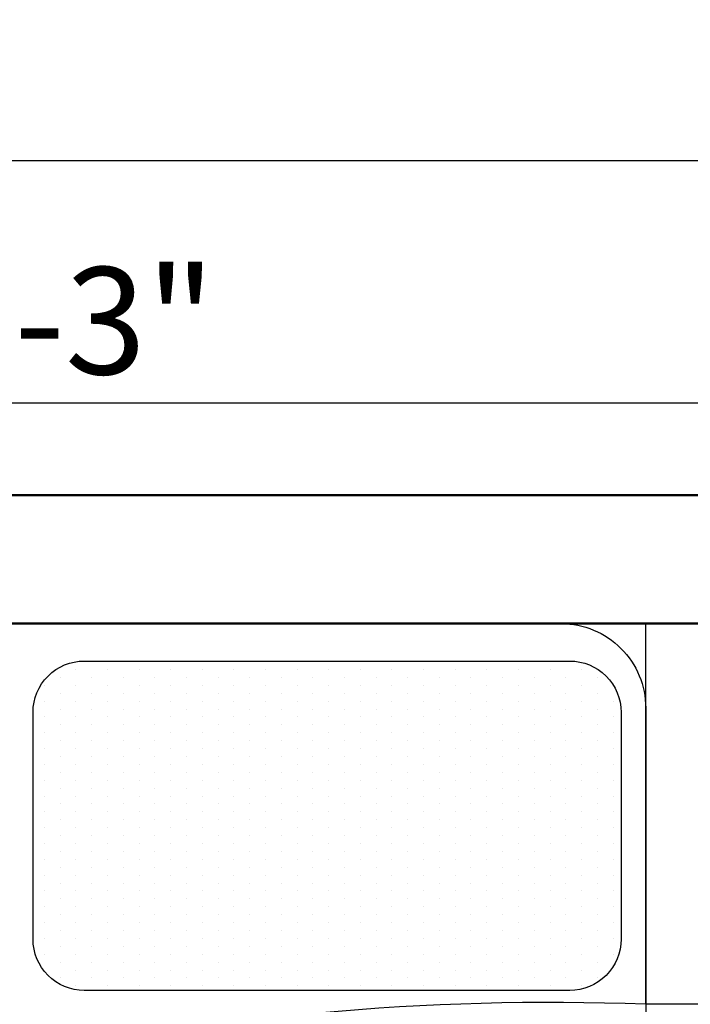
# Model space of a CAD drawing. Units: inches. Extents: x 3064 to 19385, y 846 to 15425.
# Tile 78 of 108: x 6708 to 6739, y 1964 to 2010. Entities that reach past the tile are written whole.
import ezdxf

# ---------------------------------------------------------------- set-up
doc = ezdxf.new("R2010")
doc.units = ezdxf.units.IN
for name, color, linetype, lineweight in [('A-ANNO-DIMS', 2, 'Continuous', 18), ('A-FLOR-FIXT', 9, 'Continuous', 18), ('A-WALL', 7, 'Continuous', 50)]:
    doc.layers.add(name, color=color, linetype=linetype, lineweight=lineweight)
doc.layers.add('BLOCK', color=6, linetype='Continuous')
doc.styles.get("Standard").update_dxf_attribs({"font": 'arial.ttf'})
doc.dimstyles.new('ISO-25', dxfattribs={"dimtxt": 9, "dimasz": 2.5, "dimexe": 1.25, "dimexo": 0.625, "dimtad": 1, "dimdec": 1, "dimlunit": 3, "dimtxsty": 'Standard', "dimcen": 2.5, "dimadec": 0, "dimazin": 0, "dimtfac": 1, "dimtdec": 1, "dimtmove": 0, "dimatfit": 3, "dimfxl": 1, "dimarcsym": 0})

# ---------------------------------------------------------------- blocks, each defined once
blk = doc.blocks.new('*X7')
at = {"color": 0}
for p, q in [((273.9375, 457.03125), (273.9375, 457.03125)), ((274.3125, 457.03125), (274.3125, 457.03125)), ((274.6875, 457.03125), (274.6875, 457.03125)), ((275.0625, 457.03125), (275.0625, 457.03125)), ((275.4375, 457.03125), (275.4375, 457.03125)), ((275.8125, 457.03125), (275.8125, 457.03125)), ((276.1875, 457.03125), (276.1875, 457.03125)), ((276.5625, 457.03125), (276.5625, 457.03125)), ((276.9375, 457.03125), (276.9375, 457.03125)), ((277.3125, 457.03125), (277.3125, 457.03125)), ((277.6875, 457.03125), (277.6875, 457.03125)), ((278.0625, 457.03125), (278.0625, 457.03125)), ((278.4375, 457.03125), (278.4375, 457.03125)), ((278.8125, 457.03125), (278.8125, 457.03125)), ((279.1875, 457.03125), (279.1875, 457.03125)), ((279.5625, 457.03125), (279.5625, 457.03125)), ((273.75, 456.9375), (273.75, 456.9375)), ((274.125, 456.9375), (274.125, 456.9375)), ((274.5, 456.9375), (274.5, 456.9375)), ((274.875, 456.9375), (274.875, 456.9375)), ((275.25, 456.9375), (275.25, 456.9375)), ((275.625, 456.9375), (275.625, 456.9375)), ((276, 456.9375), (276, 456.9375)), ((276.375, 456.9375), (276.375, 456.9375)), ((276.75, 456.9375), (276.75, 456.9375)), ((277.125, 456.9375), (277.125, 456.9375)), ((277.5, 456.9375), (277.5, 456.9375)), ((277.875, 456.9375), (277.875, 456.9375)), ((278.25, 456.9375), (278.25, 456.9375)), ((278.625, 456.9375), (278.625, 456.9375)), ((279, 456.9375), (279, 456.9375)), ((279.375, 456.9375), (279.375, 456.9375)), ((279.75, 456.9375), (279.75, 456.9375)), ((273.375, 456.75), (273.375, 456.75)), ((273.5625, 456.84375), (273.5625, 456.84375)), ((273.75, 456.75), (273.75, 456.75)), ((273.9375, 456.84375), (273.9375, 456.84375)), ((274.125, 456.75), (274.125, 456.75)), ((274.3125, 456.84375), (274.3125, 456.84375)), ((274.5, 456.75), (274.5, 456.75)), ((274.6875, 456.84375), (274.6875, 456.84375)), ((274.875, 456.75), (274.875, 456.75)), ((275.0625, 456.84375), (275.0625, 456.84375)), ((275.25, 456.75), (275.25, 456.75)), ((275.4375, 456.84375), (275.4375, 456.84375)), ((275.625, 456.75), (275.625, 456.75)), ((275.8125, 456.84375), (275.8125, 456.84375)), ((276, 456.75), (276, 456.75)), ((276.1875, 456.84375), (276.1875, 456.84375)), ((276.375, 456.75), (276.375, 456.75)), ((276.5625, 456.84375), (276.5625, 456.84375)), ((276.75, 456.75), (276.75, 456.75)), ((276.9375, 456.84375), (276.9375, 456.84375)), ((277.125, 456.75), (277.125, 456.75)), ((277.3125, 456.84375), (277.3125, 456.84375)), ((277.5, 456.75), (277.5, 456.75)), ((277.6875, 456.84375), (277.6875, 456.84375)), ((277.875, 456.75), (277.875, 456.75)), ((278.0625, 456.84375), (278.0625, 456.84375)), ((278.25, 456.75), (278.25, 456.75)), ((278.4375, 456.84375), (278.4375, 456.84375)), ((278.625, 456.75), (278.625, 456.75)), ((278.8125, 456.84375), (278.8125, 456.84375)), ((279, 456.75), (279, 456.75)), ((279.1875, 456.84375), (279.1875, 456.84375)), ((279.375, 456.75), (279.375, 456.75)), ((279.5625, 456.84375), (279.5625, 456.84375)), ((279.75, 456.75), (279.75, 456.75)), ((279.9375, 456.84375), (279.9375, 456.84375)), ((280.125, 456.75), (280.125, 456.75)), ((273.5625, 456.65625), (273.5625, 456.65625)), ((273.9375, 456.65625), (273.9375, 456.65625)), ((274.3125, 456.65625), (274.3125, 456.65625)), ((274.6875, 456.65625), (274.6875, 456.65625)), ((275.0625, 456.65625), (275.0625, 456.65625)), ((275.4375, 456.65625), (275.4375, 456.65625)), ((275.8125, 456.65625), (275.8125, 456.65625)), ((276.1875, 456.65625), (276.1875, 456.65625)), ((276.5625, 456.65625), (276.5625, 456.65625)), ((276.9375, 456.65625), (276.9375, 456.65625)), ((277.3125, 456.65625), (277.3125, 456.65625)), ((277.6875, 456.65625), (277.6875, 456.65625)), ((278.0625, 456.65625), (278.0625, 456.65625)), ((278.4375, 456.65625), (278.4375, 456.65625)), ((278.8125, 456.65625), (278.8125, 456.65625)), ((279.1875, 456.65625), (279.1875, 456.65625)), ((279.5625, 456.65625), (279.5625, 456.65625)), ((279.9375, 456.65625), (279.9375, 456.65625)), ((273.375, 456.5625), (273.375, 456.5625)), ((273.75, 456.5625), (273.75, 456.5625)), ((274.125, 456.5625), (274.125, 456.5625)), ((274.5, 456.5625), (274.5, 456.5625)), ((274.875, 456.5625), (274.875, 456.5625)), ((275.25, 456.5625), (275.25, 456.5625)), ((275.625, 456.5625), (275.625, 456.5625)), ((276, 456.5625), (276, 456.5625)), ((276.375, 456.5625), (276.375, 456.5625)), ((276.75, 456.5625), (276.75, 456.5625)), ((277.125, 456.5625), (277.125, 456.5625)), ((277.5, 456.5625), (277.5, 456.5625)), ((277.875, 456.5625), (277.875, 456.5625)), ((278.25, 456.5625), (278.25, 456.5625)), ((278.625, 456.5625), (278.625, 456.5625)), ((279, 456.5625), (279, 456.5625)), ((279.375, 456.5625), (279.375, 456.5625)), ((279.75, 456.5625), (279.75, 456.5625)), ((280.125, 456.5625), (280.125, 456.5625)), ((273.5625, 456.46875), (273.5625, 456.46875)), ((273.9375, 456.46875), (273.9375, 456.46875)), ((274.3125, 456.46875), (274.3125, 456.46875)), ((274.6875, 456.46875), (274.6875, 456.46875)), ((275.0625, 456.46875), (275.0625, 456.46875)), ((275.4375, 456.46875), (275.4375, 456.46875)), ((275.8125, 456.46875), (275.8125, 456.46875)), ((276.1875, 456.46875), (276.1875, 456.46875)), ((276.5625, 456.46875), (276.5625, 456.46875)), ((276.9375, 456.46875), (276.9375, 456.46875)), ((277.3125, 456.46875), (277.3125, 456.46875)), ((277.6875, 456.46875), (277.6875, 456.46875)), ((278.0625, 456.46875), (278.0625, 456.46875)), ((278.4375, 456.46875), (278.4375, 456.46875)), ((278.8125, 456.46875), (278.8125, 456.46875)), ((279.1875, 456.46875), (279.1875, 456.46875)), ((279.5625, 456.46875), (279.5625, 456.46875)), ((279.9375, 456.46875), (279.9375, 456.46875)), ((273.375, 456.375), (273.375, 456.375)), ((273.5625, 456.28125), (273.5625, 456.28125)), ((273.75, 456.375), (273.75, 456.375)), ((273.9375, 456.28125), (273.9375, 456.28125)), ((274.125, 456.375), (274.125, 456.375)), ((274.3125, 456.28125), (274.3125, 456.28125)), ((274.5, 456.375), (274.5, 456.375)), ((274.6875, 456.28125), (274.6875, 456.28125)), ((274.875, 456.375), (274.875, 456.375)), ((275.0625, 456.28125), (275.0625, 456.28125)), ((275.25, 456.375), (275.25, 456.375)), ((275.4375, 456.28125), (275.4375, 456.28125)), ((275.625, 456.375), (275.625, 456.375)), ((275.8125, 456.28125), (275.8125, 456.28125)), ((276, 456.375), (276, 456.375)), ((276.1875, 456.28125), (276.1875, 456.28125)), ((276.375, 456.375), (276.375, 456.375)), ((276.5625, 456.28125), (276.5625, 456.28125)), ((276.75, 456.375), (276.75, 456.375)), ((276.9375, 456.28125), (276.9375, 456.28125)), ((277.125, 456.375), (277.125, 456.375)), ((277.3125, 456.28125), (277.3125, 456.28125)), ((277.5, 456.375), (277.5, 456.375)), ((277.6875, 456.28125), (277.6875, 456.28125)), ((277.875, 456.375), (277.875, 456.375)), ((278.0625, 456.28125), (278.0625, 456.28125)), ((278.25, 456.375), (278.25, 456.375)), ((278.4375, 456.28125), (278.4375, 456.28125)), ((278.625, 456.375), (278.625, 456.375)), ((278.8125, 456.28125), (278.8125, 456.28125)), ((279, 456.375), (279, 456.375)), ((279.1875, 456.28125), (279.1875, 456.28125)), ((279.375, 456.375), (279.375, 456.375)), ((279.5625, 456.28125), (279.5625, 456.28125)), ((279.75, 456.375), (279.75, 456.375)), ((279.9375, 456.28125), (279.9375, 456.28125)), ((280.125, 456.375), (280.125, 456.375)), ((273.375, 456.1875), (273.375, 456.1875)), ((273.75, 456.1875), (273.75, 456.1875)), ((274.125, 456.1875), (274.125, 456.1875)), ((274.5, 456.1875), (274.5, 456.1875)), ((274.875, 456.1875), (274.875, 456.1875)), ((275.25, 456.1875), (275.25, 456.1875)), ((275.625, 456.1875), (275.625, 456.1875)), ((276, 456.1875), (276, 456.1875)), ((276.375, 456.1875), (276.375, 456.1875)), ((276.75, 456.1875), (276.75, 456.1875)), ((277.125, 456.1875), (277.125, 456.1875)), ((277.5, 456.1875), (277.5, 456.1875)), ((277.875, 456.1875), (277.875, 456.1875)), ((278.25, 456.1875), (278.25, 456.1875)), ((278.625, 456.1875), (278.625, 456.1875)), ((279, 456.1875), (279, 456.1875)), ((279.375, 456.1875), (279.375, 456.1875)), ((279.75, 456.1875), (279.75, 456.1875)), ((280.125, 456.1875), (280.125, 456.1875)), ((273.5625, 456.09375), (273.5625, 456.09375)), ((273.9375, 456.09375), (273.9375, 456.09375)), ((274.3125, 456.09375), (274.3125, 456.09375)), ((274.6875, 456.09375), (274.6875, 456.09375)), ((275.0625, 456.09375), (275.0625, 456.09375)), ((275.4375, 456.09375), (275.4375, 456.09375)), ((275.8125, 456.09375), (275.8125, 456.09375)), ((276.1875, 456.09375), (276.1875, 456.09375)), ((276.5625, 456.09375), (276.5625, 456.09375)), ((276.9375, 456.09375), (276.9375, 456.09375)), ((277.3125, 456.09375), (277.3125, 456.09375)), ((277.6875, 456.09375), (277.6875, 456.09375)), ((278.0625, 456.09375), (278.0625, 456.09375)), ((278.4375, 456.09375), (278.4375, 456.09375)), ((278.8125, 456.09375), (278.8125, 456.09375)), ((279.1875, 456.09375), (279.1875, 456.09375)), ((279.5625, 456.09375), (279.5625, 456.09375)), ((279.9375, 456.09375), (279.9375, 456.09375)), ((273.375, 456), (273.375, 456)), ((273.75, 456), (273.75, 456)), ((274.125, 456), (274.125, 456)), ((274.5, 456), (274.5, 456)), ((274.875, 456), (274.875, 456)), ((275.25, 456), (275.25, 456)), ((275.625, 456), (275.625, 456)), ((276, 456), (276, 456)), ((276.375, 456), (276.375, 456)), ((276.75, 456), (276.75, 456)), ((277.125, 456), (277.125, 456)), ((277.5, 456), (277.5, 456)), ((277.875, 456), (277.875, 456)), ((278.25, 456), (278.25, 456)), ((278.625, 456), (278.625, 456)), ((279, 456), (279, 456)), ((279.375, 456), (279.375, 456)), ((279.75, 456), (279.75, 456)), ((280.125, 456), (280.125, 456)), ((273.375, 455.8125), (273.375, 455.8125)), ((273.5625, 455.90625), (273.5625, 455.90625)), ((273.75, 455.8125), (273.75, 455.8125)), ((273.9375, 455.90625), (273.9375, 455.90625)), ((274.125, 455.8125), (274.125, 455.8125)), ((274.3125, 455.90625), (274.3125, 455.90625)), ((274.5, 455.8125), (274.5, 455.8125)), ((274.6875, 455.90625), (274.6875, 455.90625)), ((274.875, 455.8125), (274.875, 455.8125)), ((275.0625, 455.90625), (275.0625, 455.90625)), ((275.25, 455.8125), (275.25, 455.8125)), ((275.4375, 455.90625), (275.4375, 455.90625)), ((275.625, 455.8125), (275.625, 455.8125)), ((275.8125, 455.90625), (275.8125, 455.90625)), ((276, 455.8125), (276, 455.8125)), ((276.1875, 455.90625), (276.1875, 455.90625)), ((276.375, 455.8125), (276.375, 455.8125)), ((276.5625, 455.90625), (276.5625, 455.90625)), ((276.75, 455.8125), (276.75, 455.8125)), ((276.9375, 455.90625), (276.9375, 455.90625)), ((277.125, 455.8125), (277.125, 455.8125)), ((277.3125, 455.90625), (277.3125, 455.90625)), ((277.5, 455.8125), (277.5, 455.8125)), ((277.6875, 455.90625), (277.6875, 455.90625)), ((277.875, 455.8125), (277.875, 455.8125)), ((278.0625, 455.90625), (278.0625, 455.90625)), ((278.25, 455.8125), (278.25, 455.8125)), ((278.4375, 455.90625), (278.4375, 455.90625)), ((278.625, 455.8125), (278.625, 455.8125)), ((278.8125, 455.90625), (278.8125, 455.90625)), ((279, 455.8125), (279, 455.8125)), ((279.1875, 455.90625), (279.1875, 455.90625)), ((279.375, 455.8125), (279.375, 455.8125)), ((279.5625, 455.90625), (279.5625, 455.90625)), ((279.75, 455.8125), (279.75, 455.8125)), ((279.9375, 455.90625), (279.9375, 455.90625)), ((280.125, 455.8125), (280.125, 455.8125)), ((273.5625, 455.71875), (273.5625, 455.71875)), ((273.9375, 455.71875), (273.9375, 455.71875)), ((274.3125, 455.71875), (274.3125, 455.71875)), ((274.6875, 455.71875), (274.6875, 455.71875)), ((275.0625, 455.71875), (275.0625, 455.71875)), ((275.4375, 455.71875), (275.4375, 455.71875)), ((275.8125, 455.71875), (275.8125, 455.71875)), ((276.1875, 455.71875), (276.1875, 455.71875)), ((276.5625, 455.71875), (276.5625, 455.71875)), ((276.9375, 455.71875), (276.9375, 455.71875)), ((277.3125, 455.71875), (277.3125, 455.71875)), ((277.6875, 455.71875), (277.6875, 455.71875)), ((278.0625, 455.71875), (278.0625, 455.71875)), ((278.4375, 455.71875), (278.4375, 455.71875)), ((278.8125, 455.71875), (278.8125, 455.71875)), ((279.1875, 455.71875), (279.1875, 455.71875)), ((279.5625, 455.71875), (279.5625, 455.71875)), ((279.9375, 455.71875), (279.9375, 455.71875)), ((273.375, 455.625), (273.375, 455.625)), ((273.75, 455.625), (273.75, 455.625)), ((274.125, 455.625), (274.125, 455.625)), ((274.5, 455.625), (274.5, 455.625)), ((274.875, 455.625), (274.875, 455.625)), ((275.25, 455.625), (275.25, 455.625)), ((275.625, 455.625), (275.625, 455.625)), ((276, 455.625), (276, 455.625)), ((276.375, 455.625), (276.375, 455.625)), ((276.75, 455.625), (276.75, 455.625)), ((277.125, 455.625), (277.125, 455.625)), ((277.5, 455.625), (277.5, 455.625)), ((277.875, 455.625), (277.875, 455.625)), ((278.25, 455.625), (278.25, 455.625)), ((278.625, 455.625), (278.625, 455.625)), ((279, 455.625), (279, 455.625)), ((279.375, 455.625), (279.375, 455.625)), ((279.75, 455.625), (279.75, 455.625)), ((280.125, 455.625), (280.125, 455.625)), ((273.5625, 455.53125), (273.5625, 455.53125)), ((273.9375, 455.53125), (273.9375, 455.53125)), ((274.3125, 455.53125), (274.3125, 455.53125)), ((274.6875, 455.53125), (274.6875, 455.53125)), ((275.0625, 455.53125), (275.0625, 455.53125)), ((275.4375, 455.53125), (275.4375, 455.53125)), ((275.8125, 455.53125), (275.8125, 455.53125)), ((276.1875, 455.53125), (276.1875, 455.53125)), ((276.5625, 455.53125), (276.5625, 455.53125)), ((276.9375, 455.53125), (276.9375, 455.53125)), ((277.3125, 455.53125), (277.3125, 455.53125)), ((277.6875, 455.53125), (277.6875, 455.53125)), ((278.0625, 455.53125), (278.0625, 455.53125)), ((278.4375, 455.53125), (278.4375, 455.53125)), ((278.8125, 455.53125), (278.8125, 455.53125)), ((279.1875, 455.53125), (279.1875, 455.53125)), ((279.5625, 455.53125), (279.5625, 455.53125)), ((279.9375, 455.53125), (279.9375, 455.53125)), ((273.375, 455.4375), (273.375, 455.4375)), ((273.5625, 455.34375), (273.5625, 455.34375)), ((273.75, 455.4375), (273.75, 455.4375)), ((273.9375, 455.34375), (273.9375, 455.34375)), ((274.125, 455.4375), (274.125, 455.4375)), ((274.3125, 455.34375), (274.3125, 455.34375)), ((274.5, 455.4375), (274.5, 455.4375)), ((274.6875, 455.34375), (274.6875, 455.34375)), ((274.875, 455.4375), (274.875, 455.4375)), ((275.0625, 455.34375), (275.0625, 455.34375)), ((275.25, 455.4375), (275.25, 455.4375)), ((275.4375, 455.34375), (275.4375, 455.34375)), ((275.625, 455.4375), (275.625, 455.4375)), ((275.8125, 455.34375), (275.8125, 455.34375)), ((276, 455.4375), (276, 455.4375)), ((276.1875, 455.34375), (276.1875, 455.34375)), ((276.375, 455.4375), (276.375, 455.4375)), ((276.5625, 455.34375), (276.5625, 455.34375)), ((276.75, 455.4375), (276.75, 455.4375)), ((276.9375, 455.34375), (276.9375, 455.34375)), ((277.125, 455.4375), (277.125, 455.4375)), ((277.3125, 455.34375), (277.3125, 455.34375)), ((277.5, 455.4375), (277.5, 455.4375)), ((277.6875, 455.34375), (277.6875, 455.34375)), ((277.875, 455.4375), (277.875, 455.4375)), ((278.0625, 455.34375), (278.0625, 455.34375)), ((278.25, 455.4375), (278.25, 455.4375)), ((278.4375, 455.34375), (278.4375, 455.34375)), ((278.625, 455.4375), (278.625, 455.4375)), ((278.8125, 455.34375), (278.8125, 455.34375)), ((279, 455.4375), (279, 455.4375)), ((279.1875, 455.34375), (279.1875, 455.34375)), ((279.375, 455.4375), (279.375, 455.4375)), ((279.5625, 455.34375), (279.5625, 455.34375)), ((279.75, 455.4375), (279.75, 455.4375)), ((279.9375, 455.34375), (279.9375, 455.34375)), ((280.125, 455.4375), (280.125, 455.4375)), ((273.375, 455.25), (273.375, 455.25)), ((273.75, 455.25), (273.75, 455.25)), ((274.125, 455.25), (274.125, 455.25)), ((274.5, 455.25), (274.5, 455.25)), ((274.875, 455.25), (274.875, 455.25)), ((275.25, 455.25), (275.25, 455.25)), ((275.625, 455.25), (275.625, 455.25)), ((276, 455.25), (276, 455.25)), ((276.375, 455.25), (276.375, 455.25)), ((276.75, 455.25), (276.75, 455.25)), ((277.125, 455.25), (277.125, 455.25)), ((277.5, 455.25), (277.5, 455.25)), ((277.875, 455.25), (277.875, 455.25)), ((278.25, 455.25), (278.25, 455.25)), ((278.625, 455.25), (278.625, 455.25)), ((279, 455.25), (279, 455.25)), ((279.375, 455.25), (279.375, 455.25)), ((279.75, 455.25), (279.75, 455.25)), ((280.125, 455.25), (280.125, 455.25)), ((273.5625, 455.15625), (273.5625, 455.15625)), ((273.9375, 455.15625), (273.9375, 455.15625)), ((274.3125, 455.15625), (274.3125, 455.15625)), ((274.6875, 455.15625), (274.6875, 455.15625)), ((275.0625, 455.15625), (275.0625, 455.15625)), ((275.4375, 455.15625), (275.4375, 455.15625)), ((275.8125, 455.15625), (275.8125, 455.15625)), ((276.1875, 455.15625), (276.1875, 455.15625)), ((276.5625, 455.15625), (276.5625, 455.15625)), ((276.9375, 455.15625), (276.9375, 455.15625)), ((277.3125, 455.15625), (277.3125, 455.15625)), ((277.6875, 455.15625), (277.6875, 455.15625)), ((278.0625, 455.15625), (278.0625, 455.15625)), ((278.4375, 455.15625), (278.4375, 455.15625)), ((278.8125, 455.15625), (278.8125, 455.15625)), ((279.1875, 455.15625), (279.1875, 455.15625)), ((279.5625, 455.15625), (279.5625, 455.15625)), ((279.9375, 455.15625), (279.9375, 455.15625)), ((273.375, 455.0625), (273.375, 455.0625)), ((273.75, 455.0625), (273.75, 455.0625)), ((274.125, 455.0625), (274.125, 455.0625)), ((274.5, 455.0625), (274.5, 455.0625)), ((274.875, 455.0625), (274.875, 455.0625)), ((275.25, 455.0625), (275.25, 455.0625)), ((275.625, 455.0625), (275.625, 455.0625)), ((276, 455.0625), (276, 455.0625)), ((276.375, 455.0625), (276.375, 455.0625)), ((276.75, 455.0625), (276.75, 455.0625)), ((277.125, 455.0625), (277.125, 455.0625)), ((277.5, 455.0625), (277.5, 455.0625)), ((277.875, 455.0625), (277.875, 455.0625)), ((278.25, 455.0625), (278.25, 455.0625)), ((278.625, 455.0625), (278.625, 455.0625)), ((279, 455.0625), (279, 455.0625)), ((279.375, 455.0625), (279.375, 455.0625)), ((279.75, 455.0625), (279.75, 455.0625)), ((280.125, 455.0625), (280.125, 455.0625)), ((273.375, 454.875), (273.375, 454.875)), ((273.5625, 454.96875), (273.5625, 454.96875)), ((273.75, 454.875), (273.75, 454.875)), ((273.9375, 454.96875), (273.9375, 454.96875)), ((274.125, 454.875), (274.125, 454.875)), ((274.3125, 454.96875), (274.3125, 454.96875)), ((274.5, 454.875), (274.5, 454.875)), ((274.6875, 454.96875), (274.6875, 454.96875)), ((274.875, 454.875), (274.875, 454.875)), ((275.0625, 454.96875), (275.0625, 454.96875)), ((275.25, 454.875), (275.25, 454.875)), ((275.4375, 454.96875), (275.4375, 454.96875)), ((275.625, 454.875), (275.625, 454.875)), ((275.8125, 454.96875), (275.8125, 454.96875)), ((276, 454.875), (276, 454.875)), ((276.1875, 454.96875), (276.1875, 454.96875)), ((276.375, 454.875), (276.375, 454.875)), ((276.5625, 454.96875), (276.5625, 454.96875)), ((276.75, 454.875), (276.75, 454.875)), ((276.9375, 454.96875), (276.9375, 454.96875)), ((277.125, 454.875), (277.125, 454.875)), ((277.3125, 454.96875), (277.3125, 454.96875)), ((277.5, 454.875), (277.5, 454.875)), ((277.6875, 454.96875), (277.6875, 454.96875)), ((277.875, 454.875), (277.875, 454.875)), ((278.0625, 454.96875), (278.0625, 454.96875)), ((278.25, 454.875), (278.25, 454.875)), ((278.4375, 454.96875), (278.4375, 454.96875)), ((278.625, 454.875), (278.625, 454.875)), ((278.8125, 454.96875), (278.8125, 454.96875)), ((279, 454.875), (279, 454.875)), ((279.1875, 454.96875), (279.1875, 454.96875)), ((279.375, 454.875), (279.375, 454.875)), ((279.5625, 454.96875), (279.5625, 454.96875)), ((279.75, 454.875), (279.75, 454.875)), ((279.9375, 454.96875), (279.9375, 454.96875)), ((280.125, 454.875), (280.125, 454.875)), ((273.5625, 454.78125), (273.5625, 454.78125)), ((273.9375, 454.78125), (273.9375, 454.78125)), ((274.3125, 454.78125), (274.3125, 454.78125)), ((274.6875, 454.78125), (274.6875, 454.78125)), ((275.0625, 454.78125), (275.0625, 454.78125)), ((275.4375, 454.78125), (275.4375, 454.78125)), ((275.8125, 454.78125), (275.8125, 454.78125)), ((276.1875, 454.78125), (276.1875, 454.78125)), ((276.5625, 454.78125), (276.5625, 454.78125)), ((276.9375, 454.78125), (276.9375, 454.78125)), ((277.3125, 454.78125), (277.3125, 454.78125)), ((277.6875, 454.78125), (277.6875, 454.78125)), ((278.0625, 454.78125), (278.0625, 454.78125)), ((278.4375, 454.78125), (278.4375, 454.78125)), ((278.8125, 454.78125), (278.8125, 454.78125)), ((279.1875, 454.78125), (279.1875, 454.78125)), ((279.5625, 454.78125), (279.5625, 454.78125)), ((279.9375, 454.78125), (279.9375, 454.78125)), ((273.375, 454.6875), (273.375, 454.6875)), ((273.75, 454.6875), (273.75, 454.6875)), ((274.125, 454.6875), (274.125, 454.6875)), ((274.5, 454.6875), (274.5, 454.6875)), ((274.875, 454.6875), (274.875, 454.6875)), ((275.25, 454.6875), (275.25, 454.6875)), ((275.625, 454.6875), (275.625, 454.6875)), ((276, 454.6875), (276, 454.6875)), ((276.375, 454.6875), (276.375, 454.6875)), ((276.75, 454.6875), (276.75, 454.6875)), ((277.125, 454.6875), (277.125, 454.6875)), ((277.5, 454.6875), (277.5, 454.6875)), ((277.875, 454.6875), (277.875, 454.6875)), ((278.25, 454.6875), (278.25, 454.6875)), ((278.625, 454.6875), (278.625, 454.6875)), ((279, 454.6875), (279, 454.6875)), ((279.375, 454.6875), (279.375, 454.6875)), ((279.75, 454.6875), (279.75, 454.6875)), ((280.125, 454.6875), (280.125, 454.6875)), ((273.5625, 454.59375), (273.5625, 454.59375)), ((273.9375, 454.59375), (273.9375, 454.59375)), ((274.3125, 454.59375), (274.3125, 454.59375)), ((274.6875, 454.59375), (274.6875, 454.59375)), ((275.0625, 454.59375), (275.0625, 454.59375)), ((275.4375, 454.59375), (275.4375, 454.59375)), ((275.8125, 454.59375), (275.8125, 454.59375)), ((276.1875, 454.59375), (276.1875, 454.59375)), ((276.5625, 454.59375), (276.5625, 454.59375)), ((276.9375, 454.59375), (276.9375, 454.59375)), ((277.3125, 454.59375), (277.3125, 454.59375)), ((277.6875, 454.59375), (277.6875, 454.59375)), ((278.0625, 454.59375), (278.0625, 454.59375)), ((278.4375, 454.59375), (278.4375, 454.59375)), ((278.8125, 454.59375), (278.8125, 454.59375)), ((279.1875, 454.59375), (279.1875, 454.59375)), ((279.5625, 454.59375), (279.5625, 454.59375)), ((279.9375, 454.59375), (279.9375, 454.59375)), ((273.375, 454.5), (273.375, 454.5)), ((273.5625, 454.40625), (273.5625, 454.40625)), ((273.75, 454.5), (273.75, 454.5)), ((273.9375, 454.40625), (273.9375, 454.40625)), ((274.125, 454.5), (274.125, 454.5)), ((274.3125, 454.40625), (274.3125, 454.40625)), ((274.5, 454.5), (274.5, 454.5)), ((274.6875, 454.40625), (274.6875, 454.40625)), ((274.875, 454.5), (274.875, 454.5)), ((275.0625, 454.40625), (275.0625, 454.40625)), ((275.25, 454.5), (275.25, 454.5)), ((275.4375, 454.40625), (275.4375, 454.40625)), ((275.625, 454.5), (275.625, 454.5)), ((275.8125, 454.40625), (275.8125, 454.40625)), ((276, 454.5), (276, 454.5)), ((276.1875, 454.40625), (276.1875, 454.40625)), ((276.375, 454.5), (276.375, 454.5)), ((276.5625, 454.40625), (276.5625, 454.40625)), ((276.75, 454.5), (276.75, 454.5)), ((276.9375, 454.40625), (276.9375, 454.40625)), ((277.125, 454.5), (277.125, 454.5)), ((277.3125, 454.40625), (277.3125, 454.40625)), ((277.5, 454.5), (277.5, 454.5)), ((277.6875, 454.40625), (277.6875, 454.40625)), ((277.875, 454.5), (277.875, 454.5)), ((278.0625, 454.40625), (278.0625, 454.40625)), ((278.25, 454.5), (278.25, 454.5)), ((278.4375, 454.40625), (278.4375, 454.40625)), ((278.625, 454.5), (278.625, 454.5)), ((278.8125, 454.40625), (278.8125, 454.40625)), ((279, 454.5), (279, 454.5)), ((279.1875, 454.40625), (279.1875, 454.40625)), ((279.375, 454.5), (279.375, 454.5)), ((279.5625, 454.40625), (279.5625, 454.40625)), ((279.75, 454.5), (279.75, 454.5)), ((279.9375, 454.40625), (279.9375, 454.40625)), ((280.125, 454.5), (280.125, 454.5)), ((273.375, 454.3125), (273.375, 454.3125)), ((273.75, 454.3125), (273.75, 454.3125)), ((274.125, 454.3125), (274.125, 454.3125)), ((274.5, 454.3125), (274.5, 454.3125)), ((274.875, 454.3125), (274.875, 454.3125)), ((275.25, 454.3125), (275.25, 454.3125)), ((275.625, 454.3125), (275.625, 454.3125)), ((276, 454.3125), (276, 454.3125)), ((276.375, 454.3125), (276.375, 454.3125)), ((276.75, 454.3125), (276.75, 454.3125)), ((277.125, 454.3125), (277.125, 454.3125)), ((277.5, 454.3125), (277.5, 454.3125)), ((277.875, 454.3125), (277.875, 454.3125)), ((278.25, 454.3125), (278.25, 454.3125)), ((278.625, 454.3125), (278.625, 454.3125)), ((279, 454.3125), (279, 454.3125)), ((279.375, 454.3125), (279.375, 454.3125)), ((279.75, 454.3125), (279.75, 454.3125)), ((280.125, 454.3125), (280.125, 454.3125)), ((273.5625, 454.21875), (273.5625, 454.21875)), ((273.9375, 454.21875), (273.9375, 454.21875)), ((274.3125, 454.21875), (274.3125, 454.21875)), ((274.6875, 454.21875), (274.6875, 454.21875)), ((275.0625, 454.21875), (275.0625, 454.21875)), ((275.4375, 454.21875), (275.4375, 454.21875)), ((275.8125, 454.21875), (275.8125, 454.21875)), ((276.1875, 454.21875), (276.1875, 454.21875)), ((276.5625, 454.21875), (276.5625, 454.21875)), ((276.9375, 454.21875), (276.9375, 454.21875)), ((277.3125, 454.21875), (277.3125, 454.21875)), ((277.6875, 454.21875), (277.6875, 454.21875)), ((278.0625, 454.21875), (278.0625, 454.21875)), ((278.4375, 454.21875), (278.4375, 454.21875)), ((278.8125, 454.21875), (278.8125, 454.21875)), ((279.1875, 454.21875), (279.1875, 454.21875)), ((279.5625, 454.21875), (279.5625, 454.21875)), ((279.9375, 454.21875), (279.9375, 454.21875)), ((273.375, 454.125), (273.375, 454.125)), ((273.75, 454.125), (273.75, 454.125)), ((274.125, 454.125), (274.125, 454.125)), ((274.5, 454.125), (274.5, 454.125)), ((274.875, 454.125), (274.875, 454.125)), ((275.25, 454.125), (275.25, 454.125)), ((275.625, 454.125), (275.625, 454.125)), ((276, 454.125), (276, 454.125)), ((276.375, 454.125), (276.375, 454.125)), ((276.75, 454.125), (276.75, 454.125)), ((277.125, 454.125), (277.125, 454.125)), ((277.5, 454.125), (277.5, 454.125)), ((277.875, 454.125), (277.875, 454.125)), ((278.25, 454.125), (278.25, 454.125)), ((278.625, 454.125), (278.625, 454.125)), ((279, 454.125), (279, 454.125)), ((279.375, 454.125), (279.375, 454.125)), ((279.75, 454.125), (279.75, 454.125)), ((280.125, 454.125), (280.125, 454.125)), ((273.375, 453.9375), (273.375, 453.9375)), ((273.5625, 454.03125), (273.5625, 454.03125)), ((273.75, 453.9375), (273.75, 453.9375)), ((273.9375, 454.03125), (273.9375, 454.03125)), ((274.125, 453.9375), (274.125, 453.9375)), ((274.3125, 454.03125), (274.3125, 454.03125)), ((274.5, 453.9375), (274.5, 453.9375)), ((274.6875, 454.03125), (274.6875, 454.03125)), ((274.875, 453.9375), (274.875, 453.9375)), ((275.0625, 454.03125), (275.0625, 454.03125)), ((275.25, 453.9375), (275.25, 453.9375)), ((275.4375, 454.03125), (275.4375, 454.03125)), ((275.625, 453.9375), (275.625, 453.9375)), ((275.8125, 454.03125), (275.8125, 454.03125)), ((276, 453.9375), (276, 453.9375)), ((276.1875, 454.03125), (276.1875, 454.03125)), ((276.375, 453.9375), (276.375, 453.9375)), ((276.5625, 454.03125), (276.5625, 454.03125)), ((276.75, 453.9375), (276.75, 453.9375)), ((276.9375, 454.03125), (276.9375, 454.03125)), ((277.125, 453.9375), (277.125, 453.9375)), ((277.3125, 454.03125), (277.3125, 454.03125)), ((277.5, 453.9375), (277.5, 453.9375)), ((277.6875, 454.03125), (277.6875, 454.03125)), ((277.875, 453.9375), (277.875, 453.9375)), ((278.0625, 454.03125), (278.0625, 454.03125)), ((278.25, 453.9375), (278.25, 453.9375)), ((278.4375, 454.03125), (278.4375, 454.03125)), ((278.625, 453.9375), (278.625, 453.9375)), ((278.8125, 454.03125), (278.8125, 454.03125)), ((279, 453.9375), (279, 453.9375)), ((279.1875, 454.03125), (279.1875, 454.03125)), ((279.375, 453.9375), (279.375, 453.9375)), ((279.5625, 454.03125), (279.5625, 454.03125)), ((279.75, 453.9375), (279.75, 453.9375)), ((279.9375, 454.03125), (279.9375, 454.03125)), ((280.125, 453.9375), (280.125, 453.9375)), ((273.5625, 453.84375), (273.5625, 453.84375)), ((273.9375, 453.84375), (273.9375, 453.84375)), ((274.3125, 453.84375), (274.3125, 453.84375)), ((274.6875, 453.84375), (274.6875, 453.84375)), ((275.0625, 453.84375), (275.0625, 453.84375)), ((275.4375, 453.84375), (275.4375, 453.84375)), ((275.8125, 453.84375), (275.8125, 453.84375)), ((276.1875, 453.84375), (276.1875, 453.84375)), ((276.5625, 453.84375), (276.5625, 453.84375)), ((276.9375, 453.84375), (276.9375, 453.84375)), ((277.3125, 453.84375), (277.3125, 453.84375)), ((277.6875, 453.84375), (277.6875, 453.84375)), ((278.0625, 453.84375), (278.0625, 453.84375)), ((278.4375, 453.84375), (278.4375, 453.84375)), ((278.8125, 453.84375), (278.8125, 453.84375)), ((279.1875, 453.84375), (279.1875, 453.84375)), ((279.5625, 453.84375), (279.5625, 453.84375)), ((279.9375, 453.84375), (279.9375, 453.84375)), ((273.375, 453.75), (273.375, 453.75)), ((273.75, 453.75), (273.75, 453.75)), ((274.125, 453.75), (274.125, 453.75)), ((274.5, 453.75), (274.5, 453.75)), ((274.875, 453.75), (274.875, 453.75)), ((275.25, 453.75), (275.25, 453.75)), ((275.625, 453.75), (275.625, 453.75)), ((276, 453.75), (276, 453.75)), ((276.375, 453.75), (276.375, 453.75)), ((276.75, 453.75), (276.75, 453.75)), ((277.125, 453.75), (277.125, 453.75)), ((277.5, 453.75), (277.5, 453.75)), ((277.875, 453.75), (277.875, 453.75)), ((278.25, 453.75), (278.25, 453.75)), ((278.625, 453.75), (278.625, 453.75)), ((279, 453.75), (279, 453.75)), ((279.375, 453.75), (279.375, 453.75)), ((279.75, 453.75), (279.75, 453.75)), ((280.125, 453.75), (280.125, 453.75)), ((273.5625, 453.65625), (273.5625, 453.65625)), ((273.9375, 453.65625), (273.9375, 453.65625)), ((274.3125, 453.65625), (274.3125, 453.65625)), ((274.6875, 453.65625), (274.6875, 453.65625)), ((275.0625, 453.65625), (275.0625, 453.65625)), ((275.4375, 453.65625), (275.4375, 453.65625)), ((275.8125, 453.65625), (275.8125, 453.65625)), ((276.1875, 453.65625), (276.1875, 453.65625)), ((276.5625, 453.65625), (276.5625, 453.65625)), ((276.9375, 453.65625), (276.9375, 453.65625)), ((277.3125, 453.65625), (277.3125, 453.65625)), ((277.6875, 453.65625), (277.6875, 453.65625)), ((278.0625, 453.65625), (278.0625, 453.65625)), ((278.4375, 453.65625), (278.4375, 453.65625)), ((278.8125, 453.65625), (278.8125, 453.65625)), ((279.1875, 453.65625), (279.1875, 453.65625)), ((279.5625, 453.65625), (279.5625, 453.65625)), ((279.9375, 453.65625), (279.9375, 453.65625)), ((273.375, 453.5625), (273.375, 453.5625)), ((273.5625, 453.46875), (273.5625, 453.46875)), ((273.75, 453.5625), (273.75, 453.5625)), ((273.9375, 453.46875), (273.9375, 453.46875)), ((274.125, 453.5625), (274.125, 453.5625)), ((274.3125, 453.46875), (274.3125, 453.46875)), ((274.5, 453.5625), (274.5, 453.5625)), ((274.6875, 453.46875), (274.6875, 453.46875)), ((274.875, 453.5625), (274.875, 453.5625)), ((275.0625, 453.46875), (275.0625, 453.46875)), ((275.25, 453.5625), (275.25, 453.5625)), ((275.4375, 453.46875), (275.4375, 453.46875)), ((275.625, 453.5625), (275.625, 453.5625)), ((275.8125, 453.46875), (275.8125, 453.46875)), ((276, 453.5625), (276, 453.5625)), ((276.1875, 453.46875), (276.1875, 453.46875)), ((276.375, 453.5625), (276.375, 453.5625)), ((276.5625, 453.46875), (276.5625, 453.46875)), ((276.75, 453.5625), (276.75, 453.5625)), ((276.9375, 453.46875), (276.9375, 453.46875)), ((277.125, 453.5625), (277.125, 453.5625)), ((277.3125, 453.46875), (277.3125, 453.46875)), ((277.5, 453.5625), (277.5, 453.5625)), ((277.6875, 453.46875), (277.6875, 453.46875)), ((277.875, 453.5625), (277.875, 453.5625)), ((278.0625, 453.46875), (278.0625, 453.46875)), ((278.25, 453.5625), (278.25, 453.5625)), ((278.4375, 453.46875), (278.4375, 453.46875)), ((278.625, 453.5625), (278.625, 453.5625)), ((278.8125, 453.46875), (278.8125, 453.46875)), ((279, 453.5625), (279, 453.5625)), ((279.1875, 453.46875), (279.1875, 453.46875)), ((279.375, 453.5625), (279.375, 453.5625)), ((279.5625, 453.46875), (279.5625, 453.46875)), ((279.75, 453.5625), (279.75, 453.5625)), ((279.9375, 453.46875), (279.9375, 453.46875)), ((280.125, 453.5625), (280.125, 453.5625)), ((273.375, 453.375), (273.375, 453.375)), ((273.75, 453.375), (273.75, 453.375)), ((274.125, 453.375), (274.125, 453.375)), ((274.5, 453.375), (274.5, 453.375)), ((274.875, 453.375), (274.875, 453.375)), ((275.25, 453.375), (275.25, 453.375)), ((275.625, 453.375), (275.625, 453.375)), ((276, 453.375), (276, 453.375)), ((276.375, 453.375), (276.375, 453.375)), ((276.75, 453.375), (276.75, 453.375)), ((277.125, 453.375), (277.125, 453.375)), ((277.5, 453.375), (277.5, 453.375)), ((277.875, 453.375), (277.875, 453.375)), ((278.25, 453.375), (278.25, 453.375)), ((278.625, 453.375), (278.625, 453.375)), ((279, 453.375), (279, 453.375)), ((279.375, 453.375), (279.375, 453.375)), ((279.75, 453.375), (279.75, 453.375)), ((273.5625, 453.28125), (273.5625, 453.28125)), ((273.9375, 453.28125), (273.9375, 453.28125)), ((274.3125, 453.28125), (274.3125, 453.28125)), ((274.6875, 453.28125), (274.6875, 453.28125)), ((275.0625, 453.28125), (275.0625, 453.28125)), ((275.4375, 453.28125), (275.4375, 453.28125)), ((275.8125, 453.28125), (275.8125, 453.28125)), ((276.1875, 453.28125), (276.1875, 453.28125)), ((276.5625, 453.28125), (276.5625, 453.28125)), ((276.9375, 453.28125), (276.9375, 453.28125)), ((277.3125, 453.28125), (277.3125, 453.28125)), ((277.6875, 453.28125), (277.6875, 453.28125)), ((278.0625, 453.28125), (278.0625, 453.28125)), ((278.4375, 453.28125), (278.4375, 453.28125)), ((278.8125, 453.28125), (278.8125, 453.28125)), ((279.1875, 453.28125), (279.1875, 453.28125)), ((279.5625, 453.28125), (279.5625, 453.28125)), ((279.9375, 453.28125), (279.9375, 453.28125)), ((273.75, 453.1875), (273.75, 453.1875)), ((274.125, 453.1875), (274.125, 453.1875)), ((274.5, 453.1875), (274.5, 453.1875)), ((274.875, 453.1875), (274.875, 453.1875)), ((275.25, 453.1875), (275.25, 453.1875)), ((275.625, 453.1875), (275.625, 453.1875)), ((276, 453.1875), (276, 453.1875)), ((276.375, 453.1875), (276.375, 453.1875)), ((276.75, 453.1875), (276.75, 453.1875)), ((277.125, 453.1875), (277.125, 453.1875)), ((277.5, 453.1875), (277.5, 453.1875)), ((277.875, 453.1875), (277.875, 453.1875)), ((278.25, 453.1875), (278.25, 453.1875)), ((278.625, 453.1875), (278.625, 453.1875)), ((279, 453.1875), (279, 453.1875)), ((279.375, 453.1875), (279.375, 453.1875)), ((279.75, 453.1875), (279.75, 453.1875))]:
    blk.add_line(p, q, dxfattribs=at)
blk = doc.blocks.new('A$C52E67D0D')
at = {"layer": 'BLOCK'}
for points in [[(1901, 0), (601, 0, -0.414214), (501, 100), (501, 1700, -0.414214), (601, 1800), (1901, 1800, -0.414214), (2001, 1700), (2001, 100, -0.414214)], [(1911, 1365.1), (1335, 1365.1, -0.414214), (1274.2, 1425.9), (1274.2, 1694.8, -0.414214), (1335, 1755.7), (1911, 1755.7, -0.414214), (1971.8, 1694.8), (1971.8, 1425.9, -0.414214)]]:
    blk.add_lwpolyline(points, format="xyb", close=True, dxfattribs=at)
blk.add_lwpolyline([(2001, 1348.6), (2001, 1799.6), (2502, 1799.6), (2502, 1348.6)], close=True, dxfattribs=at)
blk.add_arc((1888.6, -1664.5), 3015.3, 87.8642, 117.4001, dxfattribs=at)
at = {"layer": 'BLOCK', "xscale": 100, "yscale": 100, "zscale": 100}
blk.add_blockref('*X7', (-26050, -43948.2), dxfattribs=at)
blk = doc.blocks.new('*D344')
at = {"layer": 'A-ANNO-DIMS', "color": 0, "lineweight": -2, "transparency": 16777216}
for p, q in [((6610.034, 1988.614), (6610.034, 1993.551)), ((6805.034, 1988.614), (6805.034, 1993.551)), ((6612.534, 1992.301), (6802.534, 1992.301))]:
    blk.add_line(p, q, dxfattribs=at)
at = {"layer": 'A-ANNO-DIMS', "color": 0, "transparency": 16777216}
for points in [[(6612.534, 1992.718), (6612.534, 1991.884), (6610.034, 1992.301)], [(6802.534, 1992.718), (6802.534, 1991.884), (6805.034, 1992.301)]]:
    blk.add_solid(points, dxfattribs=at)
at = {"layer": 'Defpoints', "color": 0, "transparency": 16777216}
for p in [(6805.034, 1992.301), (6610.034, 1987.989), (6805.034, 1987.989)]:
    blk.add_point(p, dxfattribs=at)
at = {"layer": 'A-ANNO-DIMS', "color": 0, "transparency": 16777216, "insert": (6707.534, 1995.481), "char_height": 5, "attachment_point": 5}
blk.add_mtext('16\'-3"', dxfattribs=at)
blk = doc.blocks.new('*D340')
at = {"layer": 'A-ANNO-DIMS', "color": 0, "lineweight": -2, "transparency": 16777216}
for p, q in [((6469.034, 1988.614), (6469.034, 2004.848)), ((6811.034, 1988.614), (6811.034, 2004.848)), ((6808.534, 2003.598), (6471.534, 2003.598))]:
    blk.add_line(p, q, dxfattribs=at)
at = {"layer": 'A-ANNO-DIMS', "color": 0, "transparency": 16777216}
for points in [[(6471.534, 2004.015), (6471.534, 2003.182), (6469.034, 2003.598)], [(6808.534, 2004.015), (6808.534, 2003.182), (6811.034, 2003.598)]]:
    blk.add_solid(points, dxfattribs=at)
at = {"layer": 'Defpoints', "color": 0, "transparency": 16777216}
for p in [(6469.034, 2003.598), (6469.034, 1987.989), (6811.034, 1987.989)]:
    blk.add_point(p, dxfattribs=at)
at = {"layer": 'A-ANNO-DIMS', "color": 0, "transparency": 16777216, "insert": (6640.034, 2006.776), "char_height": 5, "attachment_point": 5}
blk.add_mtext('28\'-6"', dxfattribs=at)

msp = doc.modelspace()

# ---------------------------------------------------------------- linework, layer by layer
at = {"layer": 'A-WALL'}
for p, q in [((6811.034, 1987.989), (6469.034, 1987.989)), ((6805.034, 1981.989), (6610.034, 1981.989))]:
    msp.add_line(p, q, dxfattribs=at)

# ---------------------------------------------------------------- block references
at = {"layer": 'A-FLOR-FIXT', "xscale": 0.039370099999992, "yscale": 0.039370099999992, "zscale": 0.039370099999992}
msp.add_blockref('A$C52E67D0D', (6658.282, 1911.123), dxfattribs=at)

# ---------------------------------------------------------------- dimensions: what is measured, and where the dimension line sits
at = {"layer": 'A-ANNO-DIMS'}
for base, p1, p2, override, picture, middle in [((6469.034, 2003.598), (6811.034, 1987.989), (6469.034, 1987.989), {"dimtxt": 5, "dimclrd": 0, "dimclre": 0, "dimclrt": 0}, '*D340', (6640.034, 2006.776)), ((6805.034, 1992.301), (6610.034, 1987.989), (6805.034, 1987.989), {"dimtxt": 5, "dimclrd": 0, "dimclre": 0, "dimclrt": 0, "dimtmove": 1}, '*D344', (6707.534, 1995.481))]:
    dim = msp.add_linear_dim(base=base, p1=p1, p2=p2, dimstyle='ISO-25', override=override, dxfattribs=at)
    dim.commit()
    dim.dimension.update_dxf_attribs({"geometry": picture, "text_midpoint": middle})

doc.saveas('drawing.dxf')
